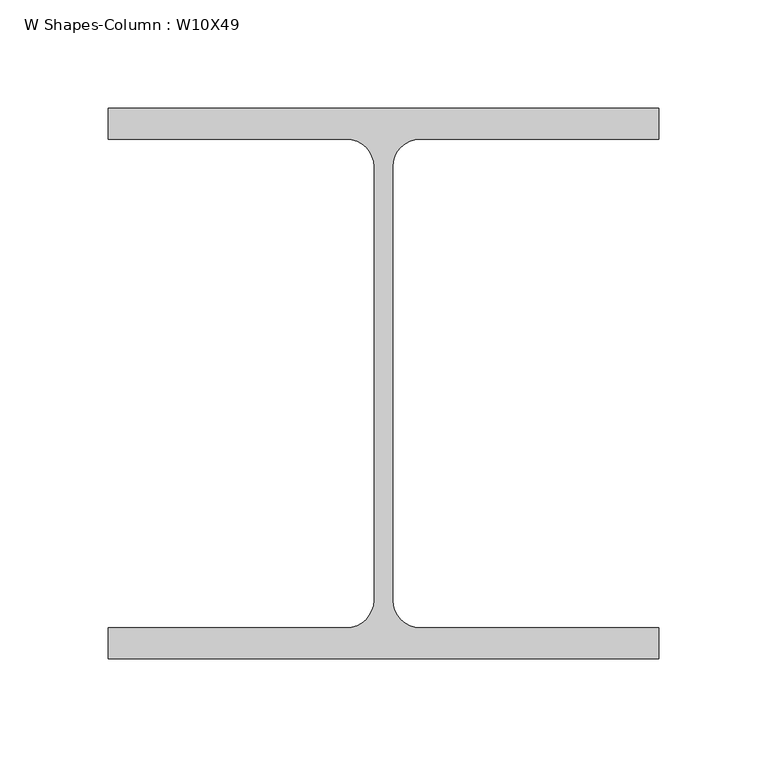
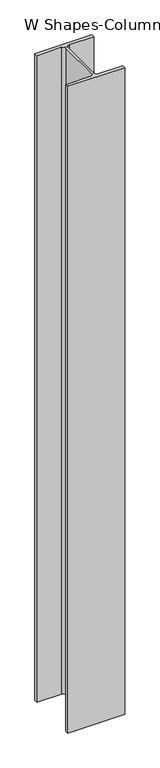
"""IFC4 building model written with IfcOpenShell, lengths in millimetres: column geometry, W Shapes-Column : W10X49."""

from ifc_helpers import new_model, si_unit, point, frame, frame_2d, origin, place, context, project, spatial, polyline, circle_curve, trimmed, segment, composite_curve, outline, extrude, source, transform, mapped, element, save


def w_shapes_column_w10x49_ceff5d29(model_context):
    return source(origin(), model_context, "Body", "SweptSolid", [
        extrude(outline(composite_curve([segment(polyline([(127.0, 127.0), (127.0, 112.776), (17.018, 112.776)]), True, "CONTINUOUS"), segment(trimmed(circle_curve(frame_2d((17.018, 100.076)), 12.7), [point((17.018, 112.776))], [point((4.318, 100.076))], True, "CARTESIAN"), True, "CONTINUOUS"), segment(polyline([(4.318, 100.076), (4.318, -100.076)]), True, "CONTINUOUS"), segment(trimmed(circle_curve(frame_2d((17.018, -100.076)), 12.7), [point((4.318, -100.076))], [point((17.018, -112.776))], True, "CARTESIAN"), True, "CONTINUOUS"), segment(polyline([(17.018, -112.776), (127.0, -112.776), (127.0, -127.0), (-127.0, -127.0), (-127.0, -112.776), (-17.018, -112.776)]), True, "CONTINUOUS"), segment(trimmed(circle_curve(frame_2d((-17.018, -100.076)), 12.7), [point((-17.018, -112.776))], [point((-4.318, -100.076))], True, "CARTESIAN"), True, "CONTINUOUS"), segment(polyline([(-4.318, -100.076), (-4.318, 100.076)]), True, "CONTINUOUS"), segment(trimmed(circle_curve(frame_2d((-17.018, 100.076)), 12.7), [point((-4.318, 100.076))], [point((-17.018, 112.776))], True, "CARTESIAN"), True, "CONTINUOUS"), segment(polyline([(-17.018, 112.776), (-127.0, 112.776), (-127.0, 127.0), (127.0, 127.0)]), True, "CONTINUOUS")], self_intersect=False)), frame((0.0, 0.0, 3048.0), z_axis=(0.0, 0.0, 1.0), x_axis=(1.0, 0.0, 0.0)), (0.0, 0.0, 1.0), 3048.0),
    ])


if __name__ == "__main__":
    model = new_model("IFC4")
    model_context = context("Model", 3, world=origin())
    ifc_project = project(units=[si_unit("LENGTHUNIT", "METRE", prefix="MILLI")], contexts=[model_context])
    site = spatial("IfcSite", under=ifc_project)
    building = spatial("IfcBuilding", under=site)
    placement = place(None, origin())
    w_shapes_column_w10x49_shape = w_shapes_column_w10x49_ceff5d29(model_context)
    element("IfcColumn", 1, ObjectType="W Shapes-Column : W10X49", at=placement, inside=building, context=model_context, shape_type="MappedRepresentation", body=[
        mapped(w_shapes_column_w10x49_shape, transform((0.0, 0.0, 0.0), x_axis=(1.0, 0.0, 0.0), y_axis=(0.0, 1.0, 0.0), z_axis=(0.0, 0.0, 1.0))),
    ])
    save(model, "model.ifc")

# Revit data of these elements
# Type "W Shapes-Column : W10X49"
#   Section Name Key = "W10x49"
#   Assembly Code = "B10"
#   Width = 10.000"
#   Web Thickness = 0.340"
#   Web Fillet = 0.500"
#   Warping Constant = 2070.00 in⁶
#   Torsional Moment of Inertia = 1.39 in⁴
#   Section Area = 14.40 in²
#   Plastic Modulus weak axis = 28.30 in³
#   Plastic Modulus strong axis = 60.40 in³
#   Perimeter = 58.50 ft²/ft
#   Nominal Weight = 49.00 lbf/ft
#   Moment of Inertia weak axis = 93.40 in⁴
#   Moment of Inertia strong axis = 272.00 in⁴
#   Height = 10.000"
#   Flange Thickness = 0.560"
#   Elastic Modulus weak axis = 18.70 in³
#   Elastic Modulus strong axis = 54.60 in³
#   Centroid Vertical = 5.000"
#   Centroid Horizontal = 5.000"
#   Bolt Spacing = 0' - 5 1/2"
#   Structural Material [instance default] = Steel ASTM A992
#   Principal Axes Angle = 0
# Element 1 (IfcColumn, "W Shapes-Column : W10X49")
#   Materials on its faces: "Steel ASTM A992"
# Materials
#   "Steel ASTM A992": class "Metal", colour RGB 199 199 199, transparency 0, Description = "Structural steel 50ksi", Cost = 0
